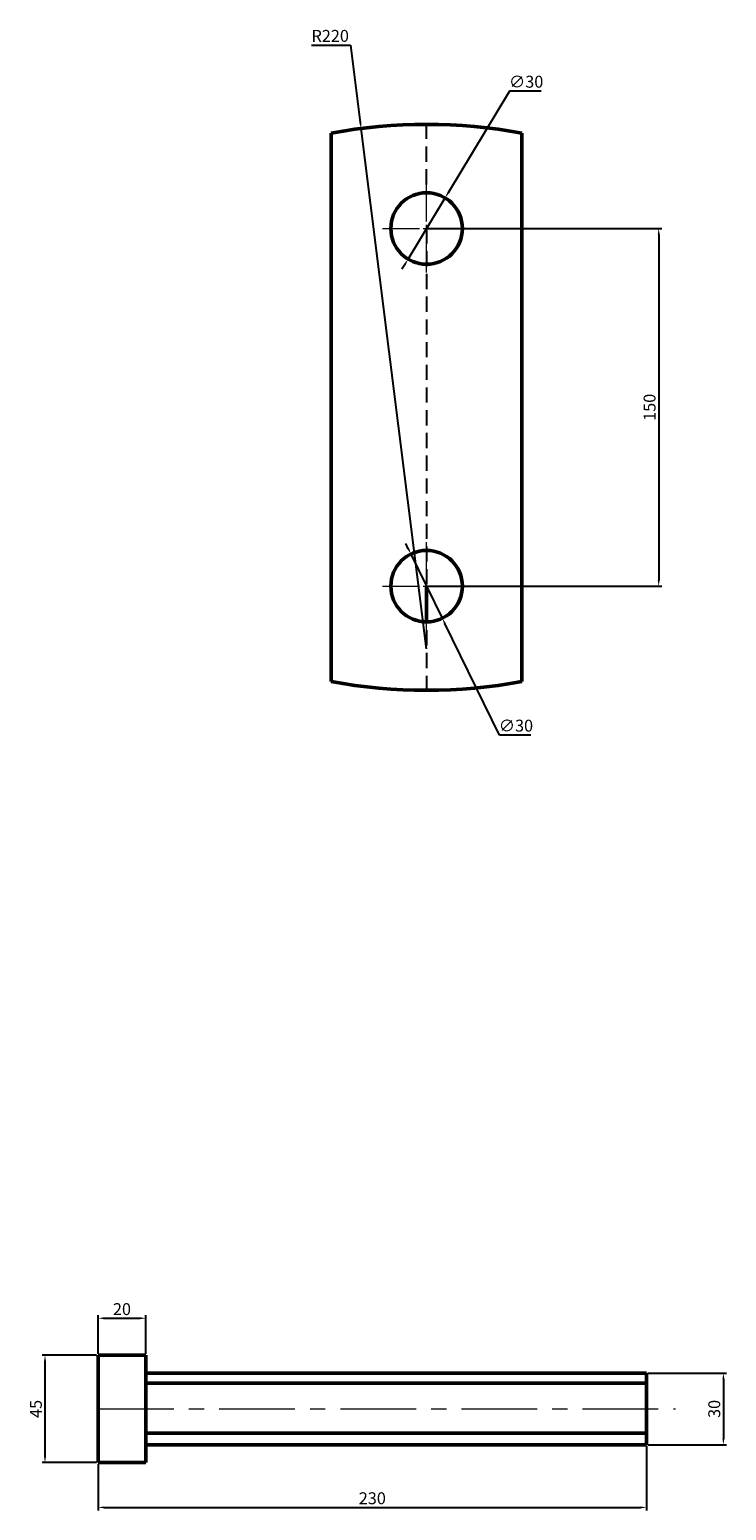
# Model space of a CAD drawing. Units: millimetres. Extents: x 1084 to 2343, y 1141 to 1965.
# Tile 3 of 4: x 1663 to 1955, y 1316 to 1937. Entities that reach past the tile are written whole.
import ezdxf

# ---------------------------------------------------------------- set-up
doc = ezdxf.new("R2010")
doc.units = ezdxf.units.MM
doc.linetypes.add('CENTER', pattern=[50.8, 31.75, -6.35, 6.35, -6.35])
doc.linetypes.add('HIDDEN', pattern=[9.525, 6.35, -3.175])
for name, color, linetype, lineweight in [('M-CNTR', 1, 'CENTER', 18), ('M-DIMS', 2, 'Continuous', 25), ('M-HIDN', 8, 'HIDDEN', 25), ('M-OUTL', 7, 'Continuous', 50)]:
    doc.layers.add(name, color=color, linetype=linetype, lineweight=lineweight)
doc.styles.get("Standard").update_dxf_attribs({"font": 'arial.ttf'})
doc.dimstyles.new('ISO-25', dxfattribs={"dimtxt": 5, "dimasz": 2.5, "dimexe": 1.25, "dimexo": 0.625, "dimtad": 1, "dimtoh": 1, "dimdec": 0, "dimtxsty": 'Standard', "dimcen": 2.5, "dimadec": 0, "dimazin": 0, "dimtfac": 1, "dimtdec": 0, "dimtmove": 0, "dimatfit": 3, "dimfxl": 1, "dimarcsym": 0})

# ---------------------------------------------------------------- blocks, each defined once
blk = doc.blocks.new('*U15')
at = {"layer": 'M-CNTR', "color": 0, "transparency": 16777216}
for p, q in [((0, 3), (0, 18.5)), ((-18.5, 0), (-3, 0)), ((3, 0), (18.5, 0)), ((0, -18.5), (0, -3))]:
    blk.add_line(p, q, dxfattribs=at)
at = {"layer": 'M-CNTR', "color": 0, "linetype": 'Continuous', "transparency": 16777216}
for p, q in [((-1.5, 0), (1.5, 0)), ((0, -1.5), (0, 1.5))]:
    blk.add_line(p, q, dxfattribs=at)
blk = doc.blocks.new('*U16')
at = {"layer": 'M-CNTR', "color": 0, "transparency": 16777216}
for p, q in [((0, 3), (0, 18.5)), ((-18.5, 0), (-3, 0)), ((3, 0), (18.5, 0)), ((0, -18.5), (0, -3))]:
    blk.add_line(p, q, dxfattribs=at)
at = {"layer": 'M-CNTR', "color": 0, "linetype": 'Continuous', "transparency": 16777216}
for p, q in [((-1.5, 0), (1.5, 0)), ((0, -1.5), (0, 1.5))]:
    blk.add_line(p, q, dxfattribs=at)
blk = doc.blocks.new('*D17')
at = {"layer": 'Defpoints', "color": 0, "transparency": 16777216}
for p in [(1801.98, 1895.29), (1829.47, 1677.01)]:
    blk.add_point(p, dxfattribs=at)
at = {"layer": 'M-DIMS', "color": 0, "lineweight": -2, "transparency": 16777216}
for p, q in [((1781.13, 1930.3), (1797.57, 1930.3)), ((1797.57, 1930.3), (1801.67, 1897.77)), ((1829.47, 1677.01), (1801.98, 1895.29))]:
    blk.add_line(p, q, dxfattribs=at)
at = {"layer": 'M-DIMS', "color": 0, "transparency": 16777216}
blk.add_solid([(1802.08, 1897.82), (1801.26, 1897.72), (1801.98, 1895.29)], dxfattribs=at)
at = {"layer": 'M-DIMS', "color": 0, "transparency": 16777216, "insert": (1789.04, 1933.48), "char_height": 5, "attachment_point": 5}
blk.add_mtext('R220', dxfattribs=at)
blk = doc.blocks.new('*D18')
at = {"layer": 'Defpoints', "color": 0, "transparency": 16777216}
for p in [(1837.23, 1866.18), (1821.71, 1840.51)]:
    blk.add_point(p, dxfattribs=at)
at = {"layer": 'M-DIMS', "color": 0, "lineweight": -2, "transparency": 16777216}
for p, q in [((1864.3, 1910.94), (1838.53, 1868.32)), ((1877.51, 1910.94), (1864.3, 1910.94)), ((1821.71, 1840.51), (1837.23, 1866.18)), ((1820.42, 1838.37), (1819.12, 1836.23))]:
    blk.add_line(p, q, dxfattribs=at)
at = {"layer": 'M-DIMS', "color": 0, "transparency": 16777216}
for points in [[(1838.17, 1868.54), (1838.88, 1868.11), (1837.23, 1866.18)], [(1820.06, 1838.59), (1820.77, 1838.16), (1821.71, 1840.51)]]:
    blk.add_solid(points, dxfattribs=at)
at = {"layer": 'M-DIMS', "color": 0, "transparency": 16777216, "insert": (1871.21, 1914.26), "char_height": 5, "attachment_point": 5}
blk.add_mtext('∅30', dxfattribs=at)
blk = doc.blocks.new('*D19')
at = {"layer": 'Defpoints', "color": 0, "transparency": 16777216}
for p in [(1822.88, 1716.82), (1836.06, 1689.87)]:
    blk.add_point(p, dxfattribs=at)
at = {"layer": 'M-DIMS', "color": 0, "lineweight": -2, "transparency": 16777216}
for p, q in [((1821.79, 1719.07), (1820.69, 1721.31)), ((1822.88, 1716.82), (1836.06, 1689.87)), ((1860.01, 1640.89), (1837.16, 1687.63)), ((1873.23, 1640.89), (1860.01, 1640.89))]:
    blk.add_line(p, q, dxfattribs=at)
at = {"layer": 'M-DIMS', "color": 0, "transparency": 16777216}
for points in [[(1822.16, 1719.25), (1821.41, 1718.89), (1822.88, 1716.82)], [(1837.53, 1687.81), (1836.79, 1687.44), (1836.06, 1689.87)]]:
    blk.add_solid(points, dxfattribs=at)
at = {"layer": 'M-DIMS', "color": 0, "transparency": 16777216, "insert": (1866.93, 1644.2), "char_height": 5, "attachment_point": 5}
blk.add_mtext('∅30', dxfattribs=at)
blk = doc.blocks.new('*D20')
at = {"layer": 'Defpoints', "color": 0, "transparency": 16777216}
for p in [(1829.47, 1853.35), (1829.47, 1703.35), (1926.81, 1703.35)]:
    blk.add_point(p, dxfattribs=at)
at = {"layer": 'M-DIMS', "color": 0, "lineweight": -2, "transparency": 16777216}
for p, q in [((1830.1, 1853.35), (1928.06, 1853.35)), ((1926.81, 1850.85), (1926.81, 1705.85)), ((1830.1, 1703.35), (1928.06, 1703.35))]:
    blk.add_line(p, q, dxfattribs=at)
at = {"layer": 'M-DIMS', "color": 0, "transparency": 16777216}
for points in [[(1926.4, 1850.85), (1927.23, 1850.85), (1926.81, 1853.35)], [(1926.4, 1705.85), (1927.23, 1705.85), (1926.81, 1703.35)]]:
    blk.add_solid(points, dxfattribs=at)
at = {"layer": 'M-DIMS', "color": 0, "transparency": 16777216, "insert": (1923.63, 1778.35), "char_height": 5, "attachment_point": 5, "rotation": 90}
blk.add_mtext('150', dxfattribs=at)
blk = doc.blocks.new('*D34')
at = {"layer": 'Defpoints', "color": 0, "transparency": 16777216}
for p in [(1691.7, 1380.8), (1669.42, 1335.8), (1691.7, 1335.8)]:
    blk.add_point(p, dxfattribs=at)
at = {"layer": 'M-DIMS', "color": 0, "lineweight": -2, "transparency": 16777216}
for p, q in [((1691.07, 1380.8), (1668.17, 1380.8)), ((1669.42, 1378.3), (1669.42, 1338.3)), ((1691.07, 1335.8), (1668.17, 1335.8))]:
    blk.add_line(p, q, dxfattribs=at)
at = {"layer": 'M-DIMS', "color": 0, "transparency": 16777216}
for points in [[(1669.01, 1378.3), (1669.84, 1378.3), (1669.42, 1380.8)], [(1669.01, 1338.3), (1669.84, 1338.3), (1669.42, 1335.8)]]:
    blk.add_solid(points, dxfattribs=at)
at = {"layer": 'M-DIMS', "color": 0, "transparency": 16777216, "insert": (1666.25, 1358.3), "char_height": 5, "attachment_point": 5, "rotation": 90}
blk.add_mtext('45', dxfattribs=at)
blk = doc.blocks.new('*D35')
at = {"layer": 'Defpoints', "color": 0, "transparency": 16777216}
for p in [(1711.7, 1396.32), (1691.7, 1380.8), (1711.7, 1380.8)]:
    blk.add_point(p, dxfattribs=at)
at = {"layer": 'M-DIMS', "color": 0, "lineweight": -2, "transparency": 16777216}
for p, q in [((1691.7, 1381.43), (1691.7, 1397.57)), ((1711.7, 1381.43), (1711.7, 1397.57)), ((1694.2, 1396.32), (1709.2, 1396.32))]:
    blk.add_line(p, q, dxfattribs=at)
at = {"layer": 'M-DIMS', "color": 0, "transparency": 16777216}
for points in [[(1694.2, 1396.74), (1694.2, 1395.9), (1691.7, 1396.32)], [(1709.2, 1396.74), (1709.2, 1395.9), (1711.7, 1396.32)]]:
    blk.add_solid(points, dxfattribs=at)
at = {"layer": 'M-DIMS', "color": 0, "transparency": 16777216, "insert": (1701.7, 1399.5), "char_height": 5, "attachment_point": 5}
blk.add_mtext('20', dxfattribs=at)
blk = doc.blocks.new('*D36')
at = {"layer": 'Defpoints', "color": 0, "transparency": 16777216}
for p in [(1921.7, 1343.3), (1691.7, 1335.8), (1921.7, 1317)]:
    blk.add_point(p, dxfattribs=at)
at = {"layer": 'M-DIMS', "color": 0, "lineweight": -2, "transparency": 16777216}
for p, q in [((1921.7, 1342.68), (1921.7, 1315.75)), ((1691.7, 1335.18), (1691.7, 1315.75)), ((1694.2, 1317), (1919.2, 1317))]:
    blk.add_line(p, q, dxfattribs=at)
at = {"layer": 'M-DIMS', "color": 0, "transparency": 16777216}
for points in [[(1694.2, 1317.41), (1694.2, 1316.58), (1691.7, 1317)], [(1919.2, 1317.41), (1919.2, 1316.58), (1921.7, 1317)]]:
    blk.add_solid(points, dxfattribs=at)
at = {"layer": 'M-DIMS', "color": 0, "transparency": 16777216, "insert": (1806.7, 1320.18), "char_height": 5, "attachment_point": 5}
blk.add_mtext('230', dxfattribs=at)
blk = doc.blocks.new('*D37')
at = {"layer": 'Defpoints', "color": 0, "transparency": 16777216}
for p in [(1921.7, 1373.3), (1921.7, 1343.3), (1953.94, 1343.3)]:
    blk.add_point(p, dxfattribs=at)
at = {"layer": 'M-DIMS', "color": 0, "lineweight": -2, "transparency": 16777216}
for p, q in [((1922.32, 1373.3), (1955.19, 1373.3)), ((1953.94, 1370.8), (1953.94, 1345.8)), ((1922.32, 1343.3), (1955.19, 1343.3))]:
    blk.add_line(p, q, dxfattribs=at)
at = {"layer": 'M-DIMS', "color": 0, "transparency": 16777216}
for points in [[(1953.53, 1370.8), (1954.36, 1370.8), (1953.94, 1373.3)], [(1953.53, 1345.8), (1954.36, 1345.8), (1953.94, 1343.3)]]:
    blk.add_solid(points, dxfattribs=at)
at = {"layer": 'M-DIMS', "color": 0, "transparency": 16777216, "insert": (1950.76, 1358.3), "char_height": 5, "attachment_point": 5, "rotation": 90}
blk.add_mtext('30', dxfattribs=at)

msp = doc.modelspace()

# ---------------------------------------------------------------- linework, layer by layer
at = {"layer": 'M-CNTR'}
msp.add_line((1691.6958, 1358.3044), (1933.8529, 1358.3044), dxfattribs=at)
at = {"layer": 'M-HIDN'}
for p, q in [((1829.4725, 1871.8478), (1829.4725, 1897.0148)), ((1829.4725, 1853.3478), (1829.4725, 1703.3478)), ((1829.4725, 1684.8478), (1829.4725, 1659.6809))]:
    msp.add_line(p, q, dxfattribs=at)
at = {"layer": 'M-OUTL'}
for p, q in [((1789.4725, 1663.3478), (1789.4725, 1893.3478)), ((1869.4725, 1893.3478), (1869.4725, 1663.3478)), ((1829.4725, 1703.3478), (1829.4725, 1688.3478)), ((1691.6958, 1380.8044), (1691.6958, 1335.8044)), ((1711.6958, 1380.8044), (1691.6958, 1380.8044)), ((1711.6958, 1335.8044), (1711.6958, 1380.8044)), ((1711.6958, 1380.8044), (1711.6958, 1373.3044)), ((1711.6958, 1373.3044), (1921.6958, 1373.3044)), ((1921.6958, 1373.3044), (1921.6958, 1343.3044)), ((1711.6958, 1369.0681), (1921.6958, 1369.0681)), ((1921.6958, 1348.1353), (1711.6958, 1348.1353)), ((1921.6958, 1343.3044), (1711.6958, 1343.3044)), ((1691.6958, 1335.8044), (1711.6958, 1335.8044))]:
    msp.add_line(p, q, dxfattribs=at)
for centre in [(1829.4725, 1853.3478), (1829.4725, 1703.3478)]:
    msp.add_circle(centre, 15, dxfattribs=at)
for centre, start, end in [((1829.4725, 1677.0148), 79.5243183, 100.4756817), ((1829.4725, 1879.6809), 259.5243183, 280.4756817)]:
    msp.add_arc(centre, 220, start, end, dxfattribs=at)

# ---------------------------------------------------------------- block references
at = {"layer": 'M-CNTR'}
for name, p in [('*U15', (1829.4725, 1853.3478)), ('*U16', (1829.4725, 1703.3478))]:
    msp.add_blockref(name, p, dxfattribs=at)

# ---------------------------------------------------------------- dimensions: what is measured, and where the dimension line sits
at = {"layer": 'M-DIMS'}
dim = msp.add_radius_dim(center=(1829.4725, 1677.0148), mpoint=(1801.9809, 1895.2903), dimstyle='ISO-25', override={"dimclrd": 0, "dimclre": 0, "dimclrt": 0}, dxfattribs=at)
dim.commit()
dim.dimension.update_dxf_attribs({"geometry": '*D17', "text_midpoint": (1789.039, 1930.2995), "dimtype": 164})
for p1, p2, picture, middle in [((1821.7117, 1840.5116), (1837.2333, 1866.1841), '*D18', (1871.2134, 1910.9449)), ((1822.8833, 1716.8231), (1836.0617, 1689.8726), '*D19', (1866.9325, 1640.8872))]:
    dim = msp.add_diameter_dim_2p(p1=p1, p2=p2, dimstyle='ISO-25', override={"dimclrd": 0, "dimclre": 0, "dimclrt": 0}, dxfattribs=at)
    dim.commit()
    dim.dimension.update_dxf_attribs({"geometry": picture, "text_midpoint": middle, "dimtype": 163})
for base, p1, p2, picture, middle in [((1926.8119, 1703.3478), (1829.4725, 1853.3478), (1829.4725, 1703.3478), '*D20', (1923.6341, 1778.3478)), ((1669.4219, 1335.8044), (1691.6958, 1380.8044), (1691.6958, 1335.8044), '*D34', (1666.2543, 1358.3044)), ((1953.9444, 1343.3044), (1921.6958, 1373.3044), (1921.6958, 1343.3044), '*D37', (1950.7649, 1358.3044))]:
    dim = msp.add_linear_dim(base=base, p1=p1, p2=p2, angle=90, dimstyle='ISO-25', override={"dimclrd": 0, "dimclre": 0, "dimclrt": 0}, dxfattribs=at)
    dim.commit()
    dim.dimension.update_dxf_attribs({"geometry": picture, "text_midpoint": middle})
for base, p1, p2, picture, middle in [((1711.6958, 1396.3214), (1691.6958, 1380.8044), (1711.6958, 1380.8044), '*D35', (1701.6958, 1399.4993)), ((1921.6958, 1316.9966), (1691.6958, 1335.8044), (1921.6958, 1343.3044), '*D36', (1806.6958, 1320.1762))]:
    dim = msp.add_linear_dim(base=base, p1=p1, p2=p2, dimstyle='ISO-25', override={"dimclrd": 0, "dimclre": 0, "dimclrt": 0}, dxfattribs=at)
    dim.commit()
    dim.dimension.update_dxf_attribs({"geometry": picture, "text_midpoint": middle})

doc.saveas('drawing.dxf')
